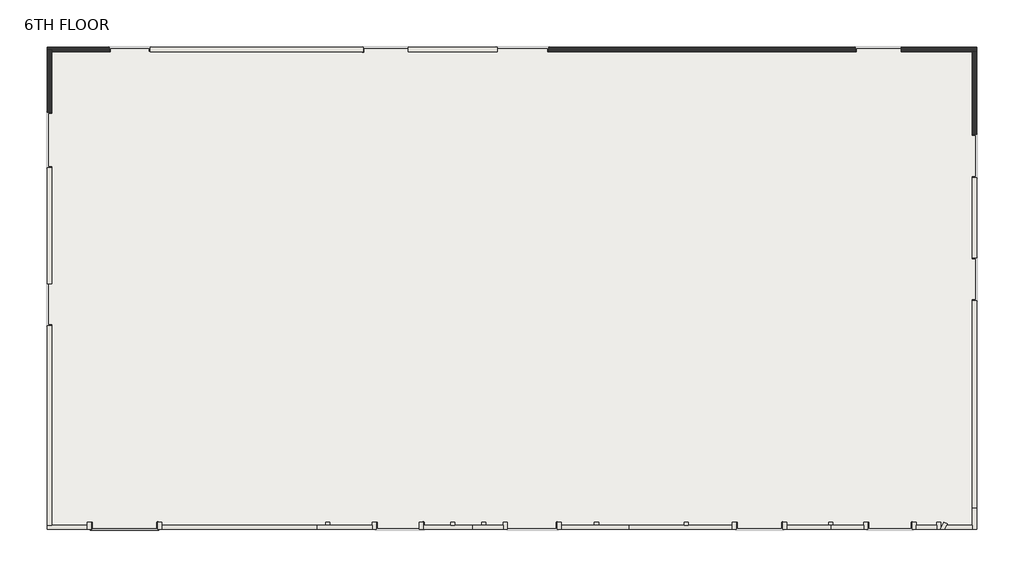
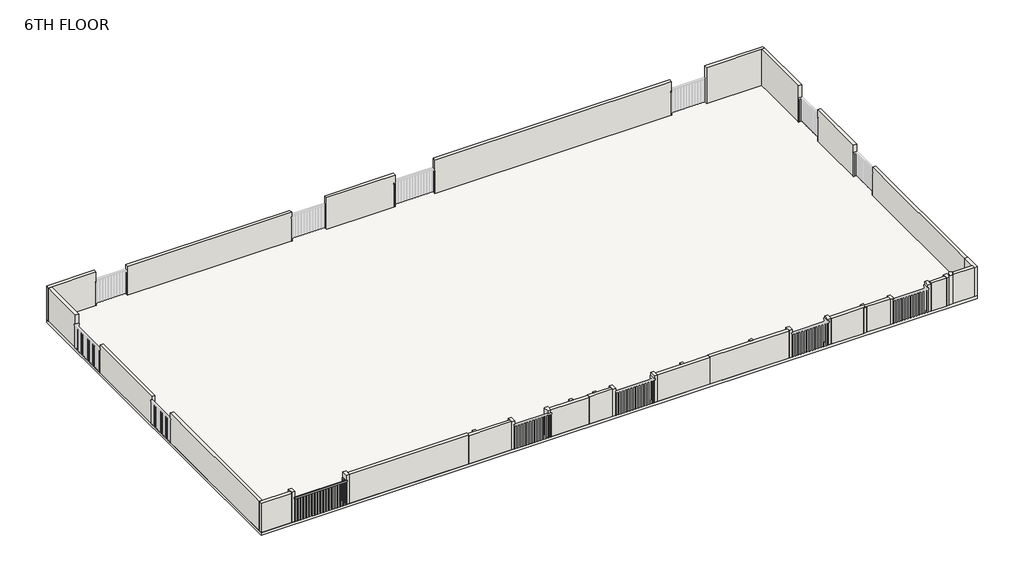
# One storey, part 1 of 3: 41 walls, 1 railing, 1 slab.
"""IFC4 building model written with IfcOpenShell, lengths in millimetres."""

from ifc_helpers import new_model, si_unit, frame, origin, place, context, project, spatial, polyline, outline, extrude, faceted_brep, element, save

model = new_model("IFC4")

# Units and contexts
model_context = context("Model", 3, world=origin())
ifc_project = project(units=[si_unit("LENGTHUNIT", "METRE", prefix="MILLI")], contexts=[model_context])

# Site, building, storey
site = spatial("IfcSite", under=ifc_project)
building = spatial("IfcBuilding", under=site)
storey = spatial("IfcBuildingStorey", under=building, Name="6TH FLOOR", Elevation=19202.4)

# Railing
placement = place(None, origin())
element("IfcRailing", 1, ObjectType="Handrail - Rectangular", at=placement, inside=storey, context=model_context, shape_type="SolidModel", body=[
    faceted_brep([(-11856.9067989, -4623.6932193, 20116.8), (-11856.9067989, -4623.6932193, 20066.0), (-11907.7067989, -4623.6932193, 20066.0), (-11907.7067989, -4623.6932193, 20116.8), (-11856.9067989, -4801.4932661, 20116.8), (-11856.9067989, -4801.4932661, 20066.0), (-11907.7067989, -4852.2932661, 20066.0), (-11907.7067989, -4852.2932661, 20116.8), (-10071.3470335, -4801.4932661, 20116.8), (-10071.3470335, -4801.4932661, 20066.0), (-10020.5470335, -4852.2932661, 20066.0), (-10020.5470335, -4852.2932661, 20116.8), (-10071.3470335, -4623.6932193, 20116.8), (-10020.5470335, -4623.6932193, 20116.8), (-10020.5470335, -4623.6932193, 20066.0), (-10071.3470335, -4623.6932193, 20066.0)], [[[0, 1, 2, 3]], [[1, 0, 4, 5]], [[2, 1, 5, 6]], [[3, 2, 6, 7]], [[0, 3, 7, 4]], [[5, 4, 8, 9]], [[6, 5, 9, 10]], [[7, 6, 10, 11]], [[4, 7, 11, 8]], [[12, 13, 14, 15]], [[9, 8, 12, 15]], [[10, 9, 15, 14]], [[11, 10, 14, 13]], [[8, 11, 13, 12]]]),
    extrude(outline(polyline([(-10036.4220335, -4633.2182661), (-10055.4720335, -4633.2182661), (-10055.4720335, -4614.1682661), (-10036.4220335, -4614.1682661), (-10036.4220335, -4633.2182661)])), frame((0.0, 0.0, 19202.4), z_axis=(0.0, 0.0, 1.0), x_axis=(1.0, 0.0, 0.0)), (0.0, 0.0, 1.0), 863.6),
    extrude(outline(polyline([(-10036.4220335, -4734.8182661), (-10055.4720335, -4734.8182661), (-10055.4720335, -4715.7682661), (-10036.4220335, -4715.7682661), (-10036.4220335, -4734.8182661)])), frame((0.0, 0.0, 19202.4), z_axis=(0.0, 0.0, 1.0), x_axis=(1.0, 0.0, 0.0)), (0.0, 0.0, 1.0), 863.6),
    extrude(outline(polyline([(-10063.0317989, -4836.4182661), (-10063.0317989, -4817.3682661), (-10043.9817989, -4817.3682661), (-10043.9817989, -4836.4182661), (-10063.0317989, -4836.4182661)])), frame((0.0, 0.0, 19202.4), z_axis=(0.0, 0.0, 1.0), x_axis=(1.0, 0.0, 0.0)), (0.0, 0.0, 1.0), 863.6),
    extrude(outline(polyline([(-10164.6317989, -4836.4182661), (-10164.6317989, -4817.3682661), (-10145.5817989, -4817.3682661), (-10145.5817989, -4836.4182661), (-10164.6317989, -4836.4182661)])), frame((0.0, 0.0, 19202.4), z_axis=(0.0, 0.0, 1.0), x_axis=(1.0, 0.0, 0.0)), (0.0, 0.0, 1.0), 863.6),
    extrude(outline(polyline([(-10266.2317989, -4836.4182661), (-10266.2317989, -4817.3682661), (-10247.1817989, -4817.3682661), (-10247.1817989, -4836.4182661), (-10266.2317989, -4836.4182661)])), frame((0.0, 0.0, 19202.4), z_axis=(0.0, 0.0, 1.0), x_axis=(1.0, 0.0, 0.0)), (0.0, 0.0, 1.0), 863.6),
    extrude(outline(polyline([(-10367.8317989, -4836.4182661), (-10367.8317989, -4817.3682661), (-10348.7817989, -4817.3682661), (-10348.7817989, -4836.4182661), (-10367.8317989, -4836.4182661)])), frame((0.0, 0.0, 19202.4), z_axis=(0.0, 0.0, 1.0), x_axis=(1.0, 0.0, 0.0)), (0.0, 0.0, 1.0), 863.6),
    extrude(outline(polyline([(-10469.4317989, -4836.4182661), (-10469.4317989, -4817.3682661), (-10450.3817989, -4817.3682661), (-10450.3817989, -4836.4182661), (-10469.4317989, -4836.4182661)])), frame((0.0, 0.0, 19202.4), z_axis=(0.0, 0.0, 1.0), x_axis=(1.0, 0.0, 0.0)), (0.0, 0.0, 1.0), 863.6),
    extrude(outline(polyline([(-10571.0317989, -4836.4182661), (-10571.0317989, -4817.3682661), (-10551.9817989, -4817.3682661), (-10551.9817989, -4836.4182661), (-10571.0317989, -4836.4182661)])), frame((0.0, 0.0, 19202.4), z_axis=(0.0, 0.0, 1.0), x_axis=(1.0, 0.0, 0.0)), (0.0, 0.0, 1.0), 863.6),
    extrude(outline(polyline([(-10672.6317989, -4836.4182661), (-10672.6317989, -4817.3682661), (-10653.5817989, -4817.3682661), (-10653.5817989, -4836.4182661), (-10672.6317989, -4836.4182661)])), frame((0.0, 0.0, 19202.4), z_axis=(0.0, 0.0, 1.0), x_axis=(1.0, 0.0, 0.0)), (0.0, 0.0, 1.0), 863.6),
    extrude(outline(polyline([(-10774.2317989, -4836.4182661), (-10774.2317989, -4817.3682661), (-10755.1817989, -4817.3682661), (-10755.1817989, -4836.4182661), (-10774.2317989, -4836.4182661)])), frame((0.0, 0.0, 19202.4), z_axis=(0.0, 0.0, 1.0), x_axis=(1.0, 0.0, 0.0)), (0.0, 0.0, 1.0), 863.6),
    extrude(outline(polyline([(-10875.8317989, -4836.4182661), (-10875.8317989, -4817.3682661), (-10856.7817989, -4817.3682661), (-10856.7817989, -4836.4182661), (-10875.8317989, -4836.4182661)])), frame((0.0, 0.0, 19202.4), z_axis=(0.0, 0.0, 1.0), x_axis=(1.0, 0.0, 0.0)), (0.0, 0.0, 1.0), 863.6),
    extrude(outline(polyline([(-10977.4317989, -4836.4182661), (-10977.4317989, -4817.3682661), (-10958.3817989, -4817.3682661), (-10958.3817989, -4836.4182661), (-10977.4317989, -4836.4182661)])), frame((0.0, 0.0, 19202.4), z_axis=(0.0, 0.0, 1.0), x_axis=(1.0, 0.0, 0.0)), (0.0, 0.0, 1.0), 863.6),
    extrude(outline(polyline([(-11079.0317989, -4836.4182661), (-11079.0317989, -4817.3682661), (-11059.9817989, -4817.3682661), (-11059.9817989, -4836.4182661), (-11079.0317989, -4836.4182661)])), frame((0.0, 0.0, 19202.4), z_axis=(0.0, 0.0, 1.0), x_axis=(1.0, 0.0, 0.0)), (0.0, 0.0, 1.0), 863.6),
    extrude(outline(polyline([(-11180.6317989, -4836.4182661), (-11180.6317989, -4817.3682661), (-11161.5817989, -4817.3682661), (-11161.5817989, -4836.4182661), (-11180.6317989, -4836.4182661)])), frame((0.0, 0.0, 19202.4), z_axis=(0.0, 0.0, 1.0), x_axis=(1.0, 0.0, 0.0)), (0.0, 0.0, 1.0), 863.6),
    extrude(outline(polyline([(-11282.2317989, -4836.4182661), (-11282.2317989, -4817.3682661), (-11263.1817989, -4817.3682661), (-11263.1817989, -4836.4182661), (-11282.2317989, -4836.4182661)])), frame((0.0, 0.0, 19202.4), z_axis=(0.0, 0.0, 1.0), x_axis=(1.0, 0.0, 0.0)), (0.0, 0.0, 1.0), 863.6),
    extrude(outline(polyline([(-11383.8317989, -4836.4182661), (-11383.8317989, -4817.3682661), (-11364.7817989, -4817.3682661), (-11364.7817989, -4836.4182661), (-11383.8317989, -4836.4182661)])), frame((0.0, 0.0, 19202.4), z_axis=(0.0, 0.0, 1.0), x_axis=(1.0, 0.0, 0.0)), (0.0, 0.0, 1.0), 863.6),
    extrude(outline(polyline([(-11485.4317989, -4836.4182661), (-11485.4317989, -4817.3682661), (-11466.3817989, -4817.3682661), (-11466.3817989, -4836.4182661), (-11485.4317989, -4836.4182661)])), frame((0.0, 0.0, 19202.4), z_axis=(0.0, 0.0, 1.0), x_axis=(1.0, 0.0, 0.0)), (0.0, 0.0, 1.0), 863.6),
    extrude(outline(polyline([(-11587.0317989, -4836.4182661), (-11587.0317989, -4817.3682661), (-11567.9817989, -4817.3682661), (-11567.9817989, -4836.4182661), (-11587.0317989, -4836.4182661)])), frame((0.0, 0.0, 19202.4), z_axis=(0.0, 0.0, 1.0), x_axis=(1.0, 0.0, 0.0)), (0.0, 0.0, 1.0), 863.6),
    extrude(outline(polyline([(-11688.6317989, -4836.4182661), (-11688.6317989, -4817.3682661), (-11669.5817989, -4817.3682661), (-11669.5817989, -4836.4182661), (-11688.6317989, -4836.4182661)])), frame((0.0, 0.0, 19202.4), z_axis=(0.0, 0.0, 1.0), x_axis=(1.0, 0.0, 0.0)), (0.0, 0.0, 1.0), 863.6),
    extrude(outline(polyline([(-11790.2317989, -4836.4182661), (-11790.2317989, -4817.3682661), (-11771.1817989, -4817.3682661), (-11771.1817989, -4836.4182661), (-11790.2317989, -4836.4182661)])), frame((0.0, 0.0, 19202.4), z_axis=(0.0, 0.0, 1.0), x_axis=(1.0, 0.0, 0.0)), (0.0, 0.0, 1.0), 863.6),
    extrude(outline(polyline([(-11891.8317989, -4817.3682193), (-11872.7817989, -4817.3682193), (-11872.7817989, -4836.4182193), (-11891.8317989, -4836.4182193), (-11891.8317989, -4817.3682193)])), frame((0.0, 0.0, 19202.4), z_axis=(0.0, 0.0, 1.0), x_axis=(1.0, 0.0, 0.0)), (0.0, 0.0, 1.0), 863.6),
    extrude(outline(polyline([(-11891.8317989, -4715.7682193), (-11872.7817989, -4715.7682193), (-11872.7817989, -4734.8182193), (-11891.8317989, -4734.8182193), (-11891.8317989, -4715.7682193)])), frame((0.0, 0.0, 19202.4), z_axis=(0.0, 0.0, 1.0), x_axis=(1.0, 0.0, 0.0)), (0.0, 0.0, 1.0), 863.6),
    extrude(outline(polyline([(-10055.4720335, -4836.4182661), (-10055.4720335, -4817.3682661), (-10036.4220335, -4817.3682661), (-10036.4220335, -4836.4182661), (-10055.4720335, -4836.4182661)])), frame((0.0, 0.0, 19202.4), z_axis=(0.0, 0.0, 1.0), x_axis=(1.0, 0.0, 0.0)), (0.0, 0.0, 1.0), 863.6),
    extrude(outline(polyline([(-11891.8317989, -4817.3682661), (-11872.7817989, -4817.3682661), (-11872.7817989, -4836.4182661), (-11891.8317989, -4836.4182661), (-11891.8317989, -4817.3682661)])), frame((0.0, 0.0, 19202.4), z_axis=(0.0, 0.0, 1.0), x_axis=(1.0, 0.0, 0.0)), (0.0, 0.0, 1.0), 863.6),
    extrude(outline(polyline([(-10036.4220335, -4642.7432193), (-10055.4720335, -4642.7432193), (-10055.4720335, -4623.6932193), (-10036.4220335, -4623.6932193), (-10036.4220335, -4642.7432193)])), frame((0.0, 0.0, 19202.4), z_axis=(0.0, 0.0, 1.0), x_axis=(1.0, 0.0, 0.0)), (0.0, 0.0, 1.0), 863.6),
    extrude(outline(polyline([(-11891.8317989, -4623.6932193), (-11872.7817989, -4623.6932193), (-11872.7817989, -4642.7432193), (-11891.8317989, -4642.7432193), (-11891.8317989, -4623.6932193)])), frame((0.0, 0.0, 19202.4), z_axis=(0.0, 0.0, 1.0), x_axis=(1.0, 0.0, 0.0)), (0.0, 0.0, 1.0), 863.6),
])

# Slab
element("IfcSlab", 2, ObjectType="LW Concrete on Metal Deck", at=placement, inside=storey, context=model_context, shape_type="SweptSolid", body=[
    extrude(outline(polyline([(12540.3012043, 8470.0067329), (12540.3012043, -4826.8932661), (-13088.8067989, -4826.8932661), (-13088.8067989, 8470.0067329), (12540.3012043, 8470.0067329)])), frame((0.0, 0.0, 19097.625), z_axis=(0.0, 0.0, 1.0), x_axis=(1.0, 0.0, 0.0)), (0.0, 0.0, 1.0), 104.775),
])

# Walls
element("IfcWall", 3, ObjectType="Generic - 4.5\"", at=placement, inside=storey, context=model_context, shape_type="Brep", body=[
    faceted_brep([(-13088.8067989, -4826.8932661, 19202.4), (-11996.6067989, -4826.8932661, 19202.4), (-11996.6067989, -4826.8932661, 20315.3417562), (-13088.8067989, -4826.8932661, 20315.3417562), (-13088.8067989, -4712.5932661, 19202.4), (-13088.8067989, -4712.5932661, 20315.3417562), (-11996.6067989, -4712.5932661, 20315.3417562), (-11996.6067989, -4712.5932661, 19202.4), (-12974.5067989, -4712.5932661, 19202.4)], [[[0, 1, 2, 3]], [[4, 5, 6, 7, 8]], [[1, 0, 4, 8, 7]], [[3, 2, 6, 5]], [[2, 1, 7, 6]], [[0, 3, 5, 4]]]),
])
element("IfcWall", 4, ObjectType="Generic - 4.5\"", at=placement, inside=storey, context=model_context, shape_type="Brep", body=[
    faceted_brep([(-11996.6067989, -4623.6932193, 19202.4), (-11996.6067989, -4712.5932661, 19202.4), (-11996.6067989, -4826.8932661, 19202.4), (-11996.6067989, -4826.8932661, 20315.3417562), (-11996.6067989, -4826.8932661, 20336.3303619), (-11996.6067989, -4623.6932193, 20336.3303619), (-11882.3067989, -4623.6932193, 19202.4), (-11882.3067989, -4623.6932193, 20336.3303619), (-11882.3067989, -4826.8932661, 20336.3303619), (-11882.3067989, -4826.8932661, 19202.4)], [[[0, 1, 2, 3, 4, 5]], [[6, 7, 8, 9]], [[2, 1, 0, 6, 9]], [[5, 4, 8, 7]], [[0, 5, 7, 6]], [[4, 3, 2, 9, 8]]]),
])
element("IfcWall", 5, ObjectType="Generic - 4.5\"", at=placement, inside=storey, context=model_context, shape_type="Brep", body=[
    faceted_brep([(11660.3143245, -4826.8932661, 19202.4), (12426.0012043, -4826.8932661, 19202.4), (12426.0012043, -4826.8932661, 20294.2617784), (12426.0012043, -4826.8932661, 20305.5196614), (11660.3143245, -4826.8932661, 20305.5196614), (11660.3143245, -4826.8932661, 20291.9342527), (11716.0621594, -4712.5932661, 19202.4), (11716.0621594, -4712.5932661, 20305.5196614), (12426.0012043, -4712.5932661, 20305.5196614), (12426.0012043, -4712.5932661, 19202.4)], [[[0, 1, 2, 3, 4, 5]], [[6, 7, 8, 9]], [[1, 0, 6, 9]], [[4, 3, 8, 7]], [[3, 2, 1, 9, 8]], [[0, 5, 4, 7, 6]]]),
])
element("IfcWall", 6, ObjectType="Generic - 4.5\"", at=placement, inside=storey, context=model_context, shape_type="Brep", body=[
    faceted_brep([(11632.2512075, -4623.6932193, 19202.4), (11533.1439227, -4826.8932661, 19202.4), (11533.1439227, -4826.8932661, 20291.9342527), (11632.2512075, -4623.6932193, 20291.9342527), (11734.983367, -4673.7990414, 19202.4), (11734.983367, -4673.7990414, 20291.9342527), (11660.3143245, -4826.8932661, 20291.9342527), (11660.3143245, -4826.8932661, 19202.4), (11716.0621594, -4712.5932661, 19202.4)], [[[0, 1, 2, 3]], [[4, 5, 6, 7, 8]], [[1, 0, 4, 8, 7]], [[3, 2, 6, 5]], [[0, 3, 5, 4]], [[2, 1, 7, 6]]]),
])
element("IfcWall", 7, ObjectType="Generic - 4.5\"", at=placement, inside=storey, context=model_context, shape_type="Brep", body=[
    faceted_brep([(12426.0012043, -4236.3432661, 19202.4), (12426.0012043, -4712.5932661, 19202.4), (12426.0012043, -4826.8932661, 19202.4), (12426.0012043, -4826.8932661, 20294.2617784), (12426.0012043, -4236.3432661, 20294.2617784), (12426.0012043, -4236.3432661, 20289.0712164), (12540.3012043, -4236.3432661, 19202.4), (12540.3012043, -4236.3432661, 20289.0712164), (12540.3012043, -4236.3432661, 20294.2617784), (12540.3012043, -4826.8932661, 20294.2617784), (12540.3012043, -4826.8932661, 19202.4)], [[[0, 1, 2, 3, 4, 5]], [[6, 7, 8, 9, 10]], [[2, 1, 0, 6, 10]], [[4, 3, 9, 8]], [[0, 5, 4, 8, 7, 6]], [[3, 2, 10, 9]]]),
])
element("IfcWall", 8, ObjectType="Generic - 4.5\"", at=placement, inside=storey, context=model_context, shape_type="SweptSolid", body=[
    extrude(outline(polyline([(-5417.4987995, -4712.5932661), (-5417.4987995, -4623.6932193), (-5303.1987995, -4623.6932193), (-5303.1987995, -4712.5932661), (-5417.4987995, -4712.5932661)])), frame((0.0, 0.0, 19202.4), z_axis=(0.0, 0.0, 1.0), x_axis=(1.0, 0.0, 0.0)), (0.0, 0.0, 1.0), 1063.0786215),
])
element("IfcWall", 9, ObjectType="Generic - 4.5\"", at=placement, inside=storey, context=model_context, shape_type="Brep", body=[
    faceted_brep([(-5663.8033402, -4826.8932661, 19202.4), (-4134.7987995, -4826.8932661, 19202.4), (-4134.7987995, -4826.8932661, 20261.5218247), (-4134.7987995, -4826.8932661, 20269.6575049), (-5663.8033402, -4826.8932661, 20269.6575049), (-5663.8033402, -4712.5932661, 19202.4), (-5663.8033402, -4712.5932661, 20269.6575049), (-4134.7987995, -4712.5932661, 20269.6575049), (-4134.7987995, -4712.5932661, 19202.4), (-5303.1987995, -4712.5932661, 19202.4), (-5417.4987995, -4712.5932661, 19202.4)], [[[0, 1, 2, 3, 4]], [[5, 6, 7, 8, 9, 10]], [[1, 0, 5, 10, 9, 8]], [[4, 3, 7, 6]], [[0, 4, 6, 5]], [[3, 2, 1, 8, 7]]]),
])
element("IfcWall", 10, ObjectType="Generic - 4.5\"", at=placement, inside=storey, context=model_context, shape_type="Brep", body=[
    faceted_brep([(-2725.0987995, -4826.8932661, 19202.4), (-1354.4417672, -4826.8932661, 19202.4), (-1354.4417672, -4826.8932661, 20218.4), (-2725.0987995, -4826.8932661, 20218.4), (-2725.0987995, -4712.5932661, 19202.4), (-2725.0987995, -4712.5932661, 20218.4), (-1354.4417672, -4712.5932661, 20218.4), (-1354.4417672, -4712.5932661, 19202.4), (-1848.7987998, -4712.5932661, 19202.4), (-1963.0987998, -4712.5932661, 19202.4)], [[[0, 1, 2, 3]], [[4, 5, 6, 7, 8, 9]], [[1, 0, 4, 9, 8, 7]], [[2, 1, 7, 6]], [[3, 2, 6, 5]], [[0, 3, 5, 4]]]),
])
element("IfcWall", 11, ObjectType="Generic - 4.5\"", at=placement, inside=storey, context=model_context, shape_type="SweptSolid", body=[
    extrude(outline(polyline([(-1963.0987998, -4712.5932661), (-1963.0987998, -4623.6932193), (-1848.7987998, -4623.6932193), (-1848.7987998, -4712.5932661), (-1963.0987998, -4712.5932661)])), frame((0.0, 0.0, 19202.4), z_axis=(0.0, 0.0, 1.0), x_axis=(1.0, 0.0, 0.0)), (0.0, 0.0, 1.0), 1029.3234006),
])
element("IfcWall", 12, ObjectType="Generic - 4.5\"", at=placement, inside=storey, context=model_context, shape_type="SweptSolid", body=[
    extrude(outline(polyline([(-1112.1987998, -4712.5932661), (-1112.1987998, -4623.6932193), (-997.8987998, -4623.6932193), (-997.8987998, -4712.5932661), (-1112.1987998, -4712.5932661)])), frame((0.0, 0.0, 19202.4), z_axis=(0.0, 0.0, 1.0), x_axis=(1.0, 0.0, 0.0)), (0.0, 0.0, 1.0), 1016.0),
])
element("IfcWall", 13, ObjectType="Generic - 4.5\"", at=placement, inside=storey, context=model_context, shape_type="SweptSolid", body=[
    extrude(outline(polyline([(1999.3012002, -4712.5932661), (1999.3012002, -4623.6932193), (2113.6012002, -4623.6932193), (2113.6012002, -4712.5932661), (1999.3012002, -4712.5932661)])), frame((0.0, 0.0, 19202.4), z_axis=(0.0, 0.0, 1.0), x_axis=(1.0, 0.0, 0.0)), (0.0, 0.0, 1.0), 1013.2250283),
])
element("IfcWall", 14, ObjectType="Generic - 4.5\"", at=placement, inside=storey, context=model_context, shape_type="SweptSolid", body=[
    extrude(outline(polyline([(4475.8012082, -4712.5932661), (4475.8012082, -4623.6932193), (4590.1012082, -4623.6932193), (4590.1012082, -4712.5932661), (4475.8012082, -4712.5932661)])), frame((0.0, 0.0, 19202.4), z_axis=(0.0, 0.0, 1.0), x_axis=(1.0, 0.0, 0.0)), (0.0, 0.0, 1.0), 1027.4591445),
])
element("IfcWall", 15, ObjectType="Generic - 4.5\"", at=placement, inside=storey, context=model_context, shape_type="Brep", body=[
    faceted_brep([(2962.6087812, -4826.8932661, 19202.4), (5802.9512082, -4826.8932661, 19202.4), (5802.9512082, -4826.8932661, 20229.8591445), (2962.6087812, -4826.8932661, 20229.8591445), (2962.6087812, -4826.8932661, 20215.6250283), (2962.6087812, -4712.5932661, 19202.4), (2962.6087812, -4712.5932661, 20215.6250283), (2962.6087812, -4712.5932661, 20229.8591445), (4475.8012082, -4712.5932661, 20229.8591445), (4590.1012082, -4712.5932661, 20229.8591445), (5802.9512082, -4712.5932661, 20229.8591445), (5802.9512082, -4712.5932661, 19202.4), (4590.1012082, -4712.5932661, 19202.4), (4475.8012082, -4712.5932661, 19202.4)], [[[0, 1, 2, 3, 4]], [[5, 6, 7, 8, 9, 10, 11, 12, 13]], [[1, 0, 5, 13, 12, 11]], [[3, 2, 10, 9, 8, 7]], [[0, 4, 3, 7, 6, 5]], [[2, 1, 11, 10]]]),
])
element("IfcWall", 16, ObjectType="Generic - 4.5\"", at=placement, inside=storey, context=model_context, shape_type="Brep", body=[
    faceted_brep([(5802.9512082, -4623.6932193, 19202.4), (5802.9512082, -4712.5932661, 19202.4), (5802.9512082, -4826.8932661, 19202.4), (5802.9512082, -4826.8932661, 20229.8591445), (5802.9512082, -4826.8932661, 20234.7822201), (5802.9512082, -4623.6932193, 20234.7822201), (5917.2512082, -4623.6932193, 19202.4), (5917.2512082, -4623.6932193, 20234.7822201), (5917.2512082, -4826.8932661, 20234.7822201), (5917.2512082, -4826.8932661, 19202.4)], [[[0, 1, 2, 3, 4, 5]], [[6, 7, 8, 9]], [[2, 1, 0, 6, 9]], [[5, 4, 8, 7]], [[0, 5, 7, 6]], [[4, 3, 2, 9, 8]]]),
])
element("IfcWall", 17, ObjectType="Generic - 4.5\"", at=placement, inside=storey, context=model_context, shape_type="Brep", body=[
    faceted_brep([(7190.3011643, -4623.6932193, 19202.4), (7190.3011643, -4826.8932661, 19202.4), (7190.3011643, -4826.8932661, 20175.2158009), (7190.3011643, -4623.6932193, 20175.2158009), (7304.6011643, -4623.6932193, 19202.4), (7304.6011643, -4623.6932193, 20175.2158009), (7304.6011643, -4712.5932661, 20175.2158009), (7304.6011643, -4826.8932661, 20175.2158009), (7304.6011643, -4826.8932661, 19202.4), (7304.6011643, -4712.5932661, 19202.4)], [[[0, 1, 2, 3]], [[4, 5, 6, 7, 8, 9]], [[1, 0, 4, 9, 8]], [[3, 2, 7, 6, 5]], [[0, 3, 5, 4]], [[2, 1, 8, 7]]]),
])
element("IfcWall", 18, ObjectType="Generic - 4.5\"", at=placement, inside=storey, context=model_context, shape_type="Brep", body=[
    faceted_brep([(7304.6011643, -4826.8932661, 19202.4), (8463.6012082, -4826.8932661, 19202.4), (8463.6012082, -4826.8932661, 20158.8159658), (8520.7512082, -4826.8932661, 20158.8159658), (8520.7512082, -4826.8932661, 20172.080309), (8520.7512082, -4826.8932661, 20175.3581334), (7304.6011643, -4826.8932661, 20175.3581334), (7304.6011643, -4712.5932661, 19202.4), (7304.6011643, -4712.5932661, 20175.3581334), (8520.7512082, -4712.5932661, 20175.3581334), (8520.7512082, -4712.5932661, 20172.080309), (8520.7512082, -4712.5932661, 20158.8159658), (8463.6012082, -4712.5932661, 20158.8159658), (8463.6012082, -4712.5932661, 19202.4)], [[[0, 1, 2, 3, 4, 5, 6]], [[7, 8, 9, 10, 11, 12, 13]], [[1, 0, 7, 13]], [[6, 5, 9, 8]], [[0, 6, 8, 7]], [[5, 4, 3, 11, 10, 9]], [[11, 3, 2, 12]], [[2, 1, 13, 12]]]),
])
element("IfcWall", 19, ObjectType="Generic - 4.5\"", at=placement, inside=storey, context=model_context, shape_type="Brep", body=[
    faceted_brep([(8463.6012082, -4623.6932193, 19202.4), (8463.6012082, -4712.5932661, 19202.4), (8463.6012082, -4826.8932661, 19202.4), (8463.6012082, -4826.8932661, 20158.8159658), (8463.6012082, -4712.5932661, 20158.8159658), (8463.6012082, -4623.6932193, 20158.8159658), (8577.9012082, -4623.6932193, 19202.4), (8577.9012082, -4623.6932193, 20158.8159658), (8577.9012082, -4712.5932661, 20158.8159658), (8577.9012082, -4826.8932661, 20158.8159658), (8577.9012082, -4826.8932661, 19202.4), (8577.9012082, -4712.5932661, 19202.4), (8520.7512082, -4826.8932661, 20158.8159658)], [[[0, 1, 2, 3, 4, 5]], [[6, 7, 8, 9, 10, 11]], [[2, 1, 0, 6, 11, 10]], [[5, 4, 3, 12, 9, 8, 7]], [[0, 5, 7, 6]], [[3, 2, 10, 9, 12]]]),
])
element("IfcWall", 20, ObjectType="Generic - 4.5\"", at=placement, inside=storey, context=model_context, shape_type="Brep", body=[
    faceted_brep([(8577.9012082, -4826.8932661, 19202.4), (9422.4512082, -4826.8932661, 19202.4), (9422.4512082, -4826.8932661, 20154.6060641), (9422.4512082, -4826.8932661, 20172.080309), (8520.7512082, -4826.8932661, 20172.080309), (8520.7512082, -4826.8932661, 20158.8159658), (8577.9012082, -4826.8932661, 20158.8159658), (8577.9012082, -4712.5932661, 19202.4), (8577.9012082, -4712.5932661, 20158.8159658), (8520.7512082, -4712.5932661, 20158.8159658), (8520.7512082, -4712.5932661, 20172.080309), (9422.4512082, -4712.5932661, 20172.080309), (9422.4512082, -4712.5932661, 19202.4)], [[[0, 1, 2, 3, 4, 5, 6]], [[7, 8, 9, 10, 11, 12]], [[1, 0, 7, 12]], [[4, 3, 11, 10]], [[3, 2, 1, 12, 11]], [[5, 4, 10, 9]], [[5, 9, 8, 6]], [[0, 6, 8, 7]]]),
])
element("IfcWall", 21, ObjectType="Generic - 4.5\"", at=placement, inside=storey, context=model_context, shape_type="Brep", body=[
    faceted_brep([(9422.4512082, -4623.6932193, 19202.4), (9422.4512082, -4712.5932661, 19202.4), (9422.4512082, -4826.8932661, 19202.4), (9422.4512082, -4826.8932661, 20154.6060641), (9422.4512082, -4623.6932193, 20154.6060641), (9536.7512082, -4623.6932193, 19202.4), (9536.7512082, -4623.6932193, 20154.6060641), (9536.7512082, -4826.8932661, 20154.6060641), (9536.7512082, -4826.8932661, 19202.4)], [[[0, 1, 2, 3, 4]], [[5, 6, 7, 8]], [[2, 1, 0, 5, 8]], [[4, 3, 7, 6]], [[0, 4, 6, 5]], [[3, 2, 8, 7]]]),
])
element("IfcWall", 22, ObjectType="Generic - 4.5\"", at=placement, inside=storey, context=model_context, shape_type="Brep", body=[
    faceted_brep([(10764.1617205, -4623.6932193, 19202.4), (10764.1617205, -4826.8932661, 19202.4), (10764.1617205, -4826.8932661, 20228.7072304), (10764.1617205, -4623.6932193, 20228.7072304), (10878.4617205, -4623.6932193, 19202.4), (10878.4617205, -4623.6932193, 20228.7072304), (10878.4617205, -4826.8932661, 20228.7072304), (10878.4617205, -4826.8932661, 19202.4), (10878.4617205, -4712.5932661, 19202.4)], [[[0, 1, 2, 3]], [[4, 5, 6, 7, 8]], [[1, 0, 4, 8, 7]], [[3, 2, 6, 5]], [[0, 3, 5, 4]], [[2, 1, 7, 6]]]),
])
element("IfcWall", 23, ObjectType="Generic - 4.5\"", at=placement, inside=storey, context=model_context, shape_type="Brep", body=[
    faceted_brep([(10878.4617205, -4826.8932661, 19202.4), (11437.2617205, -4826.8932661, 19202.4), (11437.2617205, -4826.8932661, 20251.0912221), (10878.4617205, -4826.8932661, 20251.0912221), (10878.4617205, -4826.8932661, 20228.7072304), (10878.4617205, -4712.5932661, 19202.4), (10878.4617205, -4712.5932661, 20251.0912221), (11437.2617205, -4712.5932661, 20251.0912221), (11437.2617205, -4712.5932661, 19202.4)], [[[0, 1, 2, 3, 4]], [[5, 6, 7, 8]], [[1, 0, 5, 8]], [[3, 2, 7, 6]], [[0, 4, 3, 6, 5]], [[2, 1, 8, 7]]]),
])
element("IfcWall", 24, ObjectType="Generic - 4.5\"", at=placement, inside=storey, context=model_context, shape_type="Brep", body=[
    faceted_brep([(11437.2617205, -4623.6932193, 19202.4), (11437.2617205, -4712.5932661, 19202.4), (11437.2617205, -4826.8932661, 19202.4), (11437.2617205, -4826.8932661, 20251.0912221), (11437.2617205, -4712.5932661, 20251.0912221), (11437.2617205, -4623.6932193, 20251.0912221), (11551.5617205, -4623.6932193, 19202.4), (11551.5617205, -4623.6932193, 20251.0912221), (11551.5617205, -4826.8932661, 20251.0912221), (11551.5617205, -4826.8932661, 19202.4)], [[[0, 1, 2, 3, 4, 5]], [[6, 7, 8, 9]], [[2, 1, 0, 6, 9]], [[5, 4, 3, 8, 7]], [[0, 5, 7, 6]], [[3, 2, 9, 8]]]),
])
element("IfcWall", 25, ObjectType="Generic - 4.5\"", at=placement, inside=storey, context=model_context, shape_type="Brep", body=[
    faceted_brep([(-4134.7987995, -4623.6932193, 19202.4), (-4134.7987995, -4712.5932661, 19202.4), (-4134.7987995, -4826.8932661, 19202.4), (-4134.7987995, -4826.8932661, 20261.5218247), (-4134.7987995, -4623.6932193, 20261.5218247), (-4020.4987995, -4623.6932193, 19202.4), (-4020.4987995, -4623.6932193, 20261.5218247), (-4020.4987995, -4826.8932661, 20261.5218247), (-4020.4987995, -4826.8932661, 19202.4)], [[[0, 1, 2, 3, 4]], [[5, 6, 7, 8]], [[2, 1, 0, 5, 8]], [[4, 3, 7, 6]], [[0, 4, 6, 5]], [[3, 2, 8, 7]]]),
])
element("IfcWall", 26, ObjectType="Generic - 4.5\"", at=placement, inside=storey, context=model_context, shape_type="Brep", body=[
    faceted_brep([(-2839.3987995, -4623.6932193, 19202.4), (-2839.3987995, -4826.8932661, 19202.4), (-2839.3987995, -4826.8932661, 20219.1549618), (-2839.3987995, -4623.6932193, 20219.1549618), (-2725.0987995, -4623.6932193, 19202.4), (-2725.0987995, -4623.6932193, 20219.1549618), (-2725.0987995, -4826.8932661, 20219.1549618), (-2725.0987995, -4826.8932661, 20218.4), (-2725.0987995, -4826.8932661, 19202.4), (-2725.0987995, -4712.5932661, 19202.4)], [[[0, 1, 2, 3]], [[4, 5, 6, 7, 8, 9]], [[1, 0, 4, 9, 8]], [[3, 2, 6, 5]], [[0, 3, 5, 4]], [[2, 1, 8, 7, 6]]]),
])
element("IfcWall", 27, ObjectType="Generic - 4.5\"", at=placement, inside=storey, context=model_context, shape_type="Brep", body=[
    faceted_brep([(-1354.4417672, -4826.8932661, 19202.4), (-520.5065315, -4826.8932661, 19202.4), (-520.5065315, -4826.8932661, 20226.2796817), (-520.5065315, -4826.8932661, 20233.540074), (-1354.4417672, -4826.8932661, 20233.540074), (-1354.4417672, -4826.8932661, 20218.4), (-1354.4417672, -4712.5932661, 19202.4), (-1354.4417672, -4712.5932661, 20218.4), (-1354.4417672, -4712.5932661, 20233.540074), (-520.5065315, -4712.5932661, 20233.540074), (-520.5065315, -4712.5932661, 19202.4), (-997.8987998, -4712.5932661, 19202.4), (-1112.1987998, -4712.5932661, 19202.4)], [[[0, 1, 2, 3, 4, 5]], [[6, 7, 8, 9, 10, 11, 12]], [[1, 0, 6, 12, 11, 10]], [[4, 3, 9, 8]], [[0, 5, 4, 8, 7, 6]], [[3, 2, 1, 10, 9]]]),
])
element("IfcWall", 28, ObjectType="Generic - 4.5\"", at=placement, inside=storey, context=model_context, shape_type="Brep", body=[
    faceted_brep([(-520.5065315, -4623.6932193, 19202.4), (-520.5065315, -4712.5932661, 19202.4), (-520.5065315, -4826.8932661, 19202.4), (-520.5065315, -4826.8932661, 20226.2796817), (-520.5065315, -4623.6932193, 20226.2796817), (-406.2065315, -4623.6932193, 19202.4), (-406.2065315, -4623.6932193, 20226.2796817), (-406.2065315, -4826.8932661, 20226.2796817), (-406.2065315, -4826.8932661, 19202.4)], [[[0, 1, 2, 3, 4]], [[5, 6, 7, 8]], [[2, 1, 0, 5, 8]], [[4, 3, 7, 6]], [[0, 4, 6, 5]], [[3, 2, 8, 7]]]),
])
element("IfcWall", 29, ObjectType="Generic - 4.5\"", at=placement, inside=storey, context=model_context, shape_type="Brep", body=[
    faceted_brep([(970.0932011, -4623.6932193, 19202.4), (970.0932011, -4826.8932661, 19202.4), (970.0932011, -4826.8932661, 20215.6250283), (970.0932011, -4623.6932193, 20215.6250283), (1084.3932011, -4623.6932193, 19202.4), (1084.3932011, -4623.6932193, 20215.6250283), (1084.3932011, -4712.5932661, 20215.6250283), (1084.3932011, -4826.8932661, 20215.6250283), (1084.3932011, -4826.8932661, 19202.4), (1084.3932011, -4712.5932661, 19202.4)], [[[0, 1, 2, 3]], [[4, 5, 6, 7, 8, 9]], [[1, 0, 4, 9, 8]], [[3, 2, 7, 6, 5]], [[0, 3, 5, 4]], [[2, 1, 8, 7]]]),
])
element("IfcWall", 30, ObjectType="Generic - 4.5\"", at=placement, inside=storey, context=model_context, shape_type="Brep", body=[
    faceted_brep([(1084.3932011, -4826.8932661, 19202.4), (2962.6087812, -4826.8932661, 19202.4), (2962.6087812, -4826.8932661, 20215.6250283), (1084.3932011, -4826.8932661, 20215.6250283), (1084.3932011, -4712.5932661, 19202.4), (1084.3932011, -4712.5932661, 20215.6250283), (1999.3012002, -4712.5932661, 20215.6250283), (2113.6012002, -4712.5932661, 20215.6250283), (2962.6087812, -4712.5932661, 20215.6250283), (2962.6087812, -4712.5932661, 19202.4), (2113.6012002, -4712.5932661, 19202.4), (1999.3012002, -4712.5932661, 19202.4)], [[[0, 1, 2, 3]], [[4, 5, 6, 7, 8, 9, 10, 11]], [[1, 0, 4, 11, 10, 9]], [[2, 1, 9, 8]], [[3, 2, 8, 7, 6, 5]], [[0, 3, 5, 4]]]),
])
element("IfcWall", 31, ObjectType="Generic - 4.5\"", at=placement, inside=storey, context=model_context, shape_type="Brep", body=[
    faceted_brep([(-10045.9470335, -4623.6932193, 19202.4), (-10045.9470335, -4826.8932661, 19202.4), (-10045.9470335, -4826.8932661, 20310.104535), (-10045.9470335, -4623.6932193, 20310.104535), (-9931.6470335, -4623.6932193, 19202.4), (-9931.6470335, -4623.6932193, 20310.104535), (-9931.6470335, -4712.5932661, 20310.104535), (-9931.6470335, -4826.8932661, 20310.104535), (-9931.6470335, -4826.8932661, 19202.4), (-9931.6470335, -4712.5932661, 19202.4)], [[[0, 1, 2, 3]], [[4, 5, 6, 7, 8, 9]], [[1, 0, 4, 9, 8]], [[3, 2, 7, 6, 5]], [[0, 3, 5, 4]], [[2, 1, 8, 7]]]),
])
element("IfcWall", 32, ObjectType="Generic - 4.5\"", at=placement, inside=storey, context=model_context, shape_type="Brep", body=[
    faceted_brep([(-9931.6470335, -4826.8932661, 19202.4), (-5663.8033402, -4826.8932661, 19202.4), (-5663.8033402, -4826.8932661, 20269.6575049), (-5663.8033402, -4826.8932661, 20310.104535), (-9931.6470335, -4826.8932661, 20310.104535), (-9931.6470335, -4712.5932661, 19202.4), (-9931.6470335, -4712.5932661, 20310.104535), (-5663.8033402, -4712.5932661, 20310.104535), (-5663.8033402, -4712.5932661, 20269.6575049), (-5663.8033402, -4712.5932661, 19202.4)], [[[0, 1, 2, 3, 4]], [[5, 6, 7, 8, 9]], [[1, 0, 5, 9]], [[3, 2, 1, 9, 8, 7]], [[4, 3, 7, 6]], [[0, 4, 6, 5]]]),
])
element("IfcWall", 33, ObjectType="Generic - 4.5\"", at=placement, inside=storey, context=model_context, shape_type="Brep", body=[
    faceted_brep([(-13088.8067989, 792.8567339, 19202.4), (-13088.8067989, -4712.5932661, 19202.4), (-13088.8067989, -4712.5932661, 20315.3417562), (-13088.8067989, -4712.5932661, 20316.567936), (-13088.8067989, 792.8567339, 20316.567936), (-12974.5067989, 792.8567339, 19202.4), (-12974.5067989, 792.8567339, 20316.567936), (-12974.5067989, -4712.5932661, 20316.567936), (-12974.5067989, -4712.5932661, 19202.4)], [[[0, 1, 2, 3, 4]], [[5, 6, 7, 8]], [[1, 0, 5, 8]], [[4, 3, 7, 6]], [[0, 4, 6, 5]], [[3, 2, 1, 8, 7]]]),
])
element("IfcWall", 34, ObjectType="Generic - 4.5\"", at=placement, inside=storey, context=model_context, shape_type="SweptSolid", body=[
    extrude(outline(polyline([(-12976.0338648, 5154.3604213), (-12976.0338648, 1953.9604213), (-13090.3338648, 1953.9604213), (-13090.3338648, 5154.3604213), (-12976.0338648, 5154.3604213)])), frame((0.0, 0.0, 19202.4), z_axis=(0.0, 0.0, 1.0), x_axis=(1.0, 0.0, 0.0)), (0.0, 0.0, 1.0), 1047.4413329),
])
element("IfcWall", 35, ObjectType="Generic - 4.5\"", at=placement, inside=storey, context=model_context, shape_type="SweptSolid", body=[
    extrude(outline(polyline([(-12973.9987925, 8412.8567329), (-12973.9987925, 6682.2711337), (-13088.2987925, 6682.2711337), (-13088.2987925, 8412.8567329), (-12973.9987925, 8412.8567329)])), frame((0.0, 0.0, 19202.4), z_axis=(0.0, 0.0, 1.0), x_axis=(1.0, 0.0, 0.0)), (0.0, 0.0, 1.0), 1259.0059812),
])
element("IfcWall", 36, ObjectType="Generic - 4.5\"", at=placement, inside=storey, context=model_context, shape_type="SweptSolid", body=[
    extrude(outline(polyline([(-11387.0067989, 8355.7067329), (-13088.8067989, 8355.7067329), (-13088.8067989, 8470.0067329), (-11387.0067989, 8470.0067329), (-11387.0067989, 8355.7067329)])), frame((0.0, 0.0, 19202.4), z_axis=(0.0, 0.0, 1.0), x_axis=(1.0, 0.0, 0.0)), (0.0, 0.0, 1.0), 1273.4134002),
])
element("IfcWall", 37, ObjectType="Generic - 4.5\"", at=placement, inside=storey, context=model_context, shape_type="SweptSolid", body=[
    extrude(outline(polyline([(-4382.4487992, 8355.7067329), (-10247.1817989, 8355.7067329), (-10247.1817989, 8470.0067329), (-4382.4487992, 8470.0067329), (-4382.4487992, 8355.7067329)])), frame((0.0, 0.0, 19202.4), z_axis=(0.0, 0.0, 1.0), x_axis=(1.0, 0.0, 0.0)), (0.0, 0.0, 1.0), 1083.89837),
])
element("IfcWall", 38, ObjectType="Generic - 4.5\"", at=placement, inside=storey, context=model_context, shape_type="SweptSolid", body=[
    extrude(outline(polyline([(-682.0490672, 8355.7067329), (-3139.4990672, 8355.7067329), (-3139.4990672, 8470.0067329), (-682.0490672, 8470.0067329), (-682.0490672, 8355.7067329)])), frame((0.0, 0.0, 19202.4), z_axis=(0.0, 0.0, 1.0), x_axis=(1.0, 0.0, 0.0)), (0.0, 0.0, 1.0), 1195.9732529),
])
element("IfcWall", 39, ObjectType="Generic - 4.5\"", at=placement, inside=storey, context=model_context, shape_type="SweptSolid", body=[
    extrude(outline(polyline([(9199.6932011, 8355.7067329), (741.4932011, 8355.7067329), (741.4932011, 8470.0067329), (9199.6932011, 8470.0067329), (9199.6932011, 8355.7067329)])), frame((0.0, 0.0, 19202.4), z_axis=(0.0, 0.0, 1.0), x_axis=(1.0, 0.0, 0.0)), (0.0, 0.0, 1.0), 1274.1868366),
])
element("IfcWall", 40, ObjectType="Generic - 4.5\"", at=placement, inside=storey, context=model_context, shape_type="Brep", body=[
    faceted_brep([(10462.2009401, 8355.7067329, 19202.4), (12426.0012043, 8355.7067329, 19202.4), (12540.3012043, 8355.7067329, 19202.4), (12540.3012043, 8355.7067329, 20568.1502881), (10462.2009401, 8355.7067329, 20568.1502881), (10462.2009401, 8470.0067329, 19202.4), (10462.2009401, 8470.0067329, 20568.1502881), (12540.3012043, 8470.0067329, 20568.1502881), (12540.3012043, 8470.0067329, 19202.4)], [[[0, 1, 2, 3, 4]], [[5, 6, 7, 8]], [[2, 1, 0, 5, 8]], [[4, 3, 7, 6]], [[0, 4, 6, 5]], [[3, 2, 8, 7]]]),
])
element("IfcWall", 41, ObjectType="Generic - 4.5\"", at=placement, inside=storey, context=model_context, shape_type="SweptSolid", body=[
    extrude(outline(polyline([(12426.0012043, -4236.3432661), (12426.0012043, 1478.6567334), (12540.3012043, 1478.6567334), (12540.3012043, -4236.3432661), (12426.0012043, -4236.3432661)])), frame((0.0, 0.0, 19202.4), z_axis=(0.0, 0.0, 1.0), x_axis=(1.0, 0.0, 0.0)), (0.0, 0.0, 1.0), 1086.6712164),
])
element("IfcWall", 42, ObjectType="Generic - 4.5\"", at=placement, inside=storey, context=model_context, shape_type="Brep", body=[
    faceted_brep([(12426.0012043, 8355.7067329, 19202.4), (12426.0012043, 6069.7067329, 19202.4), (12426.0012043, 6069.7067329, 20574.0), (12426.0012043, 8355.7067329, 20574.0), (12540.3012043, 8355.7067329, 19202.4), (12540.3012043, 8355.7067329, 20568.1502881), (12540.3012043, 8355.7067329, 20574.0), (12540.3012043, 6069.7067329, 20574.0), (12540.3012043, 6069.7067329, 19202.4)], [[[0, 1, 2, 3]], [[4, 5, 6, 7, 8]], [[1, 0, 4, 8]], [[2, 1, 8, 7]], [[3, 2, 7, 6]], [[0, 3, 6, 5, 4]]]),
])
element("IfcWall", 43, ObjectType="Generic - 4.5\"", at=placement, inside=storey, context=model_context, shape_type="SweptSolid", body=[
    extrude(outline(polyline([(12426.0012043, 2666.1067329), (12426.0012043, 4875.9067329), (12540.3012043, 4875.9067329), (12540.3012043, 2666.1067329), (12426.0012043, 2666.1067329)])), frame((0.0, 0.0, 19202.4), z_axis=(0.0, 0.0, 1.0), x_axis=(1.0, 0.0, 0.0)), (0.0, 0.0, 1.0), 1193.0409005),
])

save(model, "model.ifc")

# Revit data of these elements
# Type "Handrail - Rectangular"
#   Assembly Code = "C2010400"
#   built-in parameter 1008612 = 0.0416667 (stored number, unit not read)
#   built-in parameter 1008611 = 0.0416667 (stored number, unit not read)
#   built-in parameter 1008609 = 0.333333 (stored number, unit not read)
#   built-in parameter 1008604 = 0.166667 (stored number, unit not read)
#   built-in parameter 1008603 = 0.166667 (stored number, unit not read)
#   Railing Height = 3' - 0"
#   built-in parameter 1008630 = 2
#   built-in parameter 1008610 = 2
#   built-in parameter 1008618 = Baluster - Square : 3/4"
# Type "LW Concrete on Metal Deck"
#   Assembly Code = "B1010"
#   Function = 0
#   Layers, outside or top first: 0' - 4" "Concrete, Lightweight" (function 1); 0' - 0 1/8" "Metal Deck" (function 1)
# Type "Generic - 4.5\""
#   Assembly Code = "B2010"
#   Layers, outside or top first: 0' - 4 1/2" no material (function 1)
# Element 1 (IfcRailing, "Handrail - Rectangular")
#   Phase Created = New Construction
# Element 2 (IfcSlab, "LW Concrete on Metal Deck")
#   Height Offset From Level = 0' - 0"
#   Phase Created = New Construction
#   Materials on its faces: "Metal Deck", "Concrete, Lightweight"
# Element 3 (IfcWall, "Generic - 4.5\"")
#   Top Offset = -6' - 10.1834"
#   Base Offset = 0' - 0"
#   wall height = 3' - 7.8166"
#   Phase Created = New Construction
#   Base Constraint = 6TH FLOOR
#   Top Constraint = ROOF
#   Materials on its faces: "Default Wall"
# Element 4 (IfcWall, "Generic - 4.5\"")
#   Top Offset = 0' - 0"
#   Base Offset = 0' - 0"
#   Unconnected Height = 3' - 8.64293"
#   wall height = 3' - 8.64293"
#   Phase Created = New Construction
#   Base Constraint = 6TH FLOOR
#   Materials on its faces: "Default Wall"
# Element 5 (IfcWall, "Generic - 4.5\"")
#   Top Offset = -6' - 10.57009"
#   Base Offset = 0' - 0"
#   wall height = 3' - 7.42991"
#   Phase Created = New Construction
#   Base Constraint = 6TH FLOOR
#   Top Constraint = ROOF
#   Materials on its faces: "Default Wall"
# Element 6 (IfcWall, "Generic - 4.5\"")
#   Top Offset = -6' - 11.10495"
#   Base Offset = 0' - 0"
#   wall height = 3' - 6.89505"
#   Phase Created = New Construction
#   Base Constraint = 6TH FLOOR
#   Top Constraint = ROOF
#   Materials on its faces: "Default Wall"
# Element 7 (IfcWall, "Generic - 4.5\"")
#   Top Offset = -6' - 11.01332"
#   Base Offset = 0' - 0"
#   wall height = 3' - 6.98668"
#   Phase Created = New Construction
#   Base Constraint = 6TH FLOOR
#   Top Constraint = ROOF
#   Materials on its faces: "Default Wall"
# Element 8 (IfcWall, "Generic - 4.5\"")
#   Top Offset = -7' - 0.14651"
#   Base Offset = 0' - 0"
#   wall height = 3' - 5.85349"
#   Phase Created = New Construction
#   Base Constraint = 6TH FLOOR
#   Top Constraint = ROOF
#   Materials on its faces: "Default Wall"
# Element 9 (IfcWall, "Generic - 4.5\"")
#   Top Offset = -6' - 11.98199"
#   Base Offset = 0' - 0"
#   wall height = 3' - 6.01801"
#   Phase Created = New Construction
#   Base Constraint = 6TH FLOOR
#   Top Constraint = ROOF
#   Materials on its faces: "Default Wall"
# Elements 10, 12 (IfcWall, "Generic - 4.5\"")
#   Top Offset = -7' - 2"
#   Base Offset = 0' - 0"
#   wall height = 3' - 4"
#   Phase Created = New Construction
#   Base Constraint = 6TH FLOOR
#   Top Constraint = ROOF
#   Materials on its faces: "Default Wall"
# Element 11 (IfcWall, "Generic - 4.5\"")
#   Top Offset = -7' - 1.47546"
#   Base Offset = 0' - 0"
#   wall height = 3' - 4.52454"
#   Phase Created = New Construction
#   Base Constraint = 6TH FLOOR
#   Top Constraint = ROOF
#   Materials on its faces: "Default Wall"
# Elements 13, 29, 30 (IfcWall, "Generic - 4.5\"")
#   Top Offset = -7' - 2.10925"
#   Base Offset = 0' - 0"
#   wall height = 3' - 3.89075"
#   Phase Created = New Construction
#   Base Constraint = 6TH FLOOR
#   Top Constraint = ROOF
#   Materials on its faces: "Default Wall"
# Elements 14, 15 (IfcWall, "Generic - 4.5\"")
#   Top Offset = -7' - 1.54885"
#   Base Offset = 0' - 0"
#   wall height = 3' - 4.45115"
#   Phase Created = New Construction
#   Base Constraint = 6TH FLOOR
#   Top Constraint = ROOF
#   Materials on its faces: "Default Wall"
# Element 16 (IfcWall, "Generic - 4.5\"")
#   Top Offset = -7' - 1.35503"
#   Base Offset = 0' - 0"
#   wall height = 3' - 4.64497"
#   Phase Created = New Construction
#   Base Constraint = 6TH FLOOR
#   Top Constraint = ROOF
#   Materials on its faces: "Default Wall"
# Element 17 (IfcWall, "Generic - 4.5\"")
#   Top Offset = -7' - 3.70017"
#   Base Offset = 0' - 0"
#   wall height = 3' - 2.29983"
#   Phase Created = New Construction
#   Base Constraint = 6TH FLOOR
#   Top Constraint = ROOF
#   Materials on its faces: "Default Wall"
# Element 18 (IfcWall, "Generic - 4.5\"")
#   Top Offset = -7' - 3.69456"
#   Base Offset = 0' - 0"
#   wall height = 3' - 2.30544"
#   Phase Created = New Construction
#   Base Constraint = 6TH FLOOR
#   Top Constraint = ROOF
#   Materials on its faces: "Default Wall"
# Element 19 (IfcWall, "Generic - 4.5\"")
#   Top Offset = -7' - 4.34583"
#   Base Offset = 0' - 0"
#   wall height = 3' - 1.65417"
#   Phase Created = New Construction
#   Base Constraint = 6TH FLOOR
#   Top Constraint = ROOF
#   Materials on its faces: "Default Wall"
# Element 20 (IfcWall, "Generic - 4.5\"")
#   Top Offset = -7' - 3.82361"
#   Base Offset = 0' - 0"
#   wall height = 3' - 2.17639"
#   Phase Created = New Construction
#   Base Constraint = 6TH FLOOR
#   Top Constraint = ROOF
#   Materials on its faces: "Default Wall"
# Element 21 (IfcWall, "Generic - 4.5\"")
#   Top Offset = -7' - 4.51157"
#   Base Offset = 0' - 0"
#   wall height = 3' - 1.48843"
#   Phase Created = New Construction
#   Base Constraint = 6TH FLOOR
#   Top Constraint = ROOF
#   Materials on its faces: "Default Wall"
# Element 22 (IfcWall, "Generic - 4.5\"")
#   Top Offset = -7' - 1.5942"
#   Base Offset = 0' - 0"
#   wall height = 3' - 4.4058"
#   Phase Created = New Construction
#   Base Constraint = 6TH FLOOR
#   Top Constraint = ROOF
#   Materials on its faces: "Default Wall"
# Elements 23, 24 (IfcWall, "Generic - 4.5\"")
#   Top Offset = -7' - 0.71294"
#   Base Offset = 0' - 0"
#   wall height = 3' - 5.28706"
#   Phase Created = New Construction
#   Base Constraint = 6TH FLOOR
#   Top Constraint = ROOF
#   Materials on its faces: "Default Wall"
# Element 25 (IfcWall, "Generic - 4.5\"")
#   Top Offset = -7' - 0.30229"
#   Base Offset = 0' - 0"
#   wall height = 3' - 5.69771"
#   Phase Created = New Construction
#   Base Constraint = 6TH FLOOR
#   Top Constraint = ROOF
#   Materials on its faces: "Default Wall"
# Element 26 (IfcWall, "Generic - 4.5\"")
#   Top Offset = -7' - 1.97028"
#   Base Offset = 0' - 0"
#   wall height = 3' - 4.02972"
#   Phase Created = New Construction
#   Base Constraint = 6TH FLOOR
#   Top Constraint = ROOF
#   Materials on its faces: "Default Wall"
# Element 27 (IfcWall, "Generic - 4.5\"")
#   Top Offset = -7' - 1.40393"
#   Base Offset = 0' - 0"
#   wall height = 3' - 4.59607"
#   Phase Created = New Construction
#   Base Constraint = 6TH FLOOR
#   Top Constraint = ROOF
#   Materials on its faces: "Default Wall"
# Element 28 (IfcWall, "Generic - 4.5\"")
#   Top Offset = -7' - 1.68978"
#   Base Offset = 0' - 0"
#   wall height = 3' - 4.31022"
#   Phase Created = New Construction
#   Base Constraint = 6TH FLOOR
#   Top Constraint = ROOF
#   Materials on its faces: "Default Wall"
# Elements 31, 32 (IfcWall, "Generic - 4.5\"")
#   Top Offset = -6' - 10.38959"
#   Base Offset = 0' - 0"
#   wall height = 3' - 7.61041"
#   Phase Created = New Construction
#   Base Constraint = 6TH FLOOR
#   Top Constraint = ROOF
#   Materials on its faces: "Default Wall"
# Element 33 (IfcWall, "Generic - 4.5\"")
#   Top Offset = 0' - 0"
#   Base Offset = 0' - 0"
#   Unconnected Height = 3' - 7.86488"
#   wall height = 3' - 7.86488"
#   Phase Created = New Construction
#   Base Constraint = 6TH FLOOR
#   Materials on its faces: "Default Wall"
# Element 34 (IfcWall, "Generic - 4.5\"")
#   Top Offset = -7' - 0.76215"
#   Base Offset = 0' - 0"
#   wall height = 3' - 5.23785"
#   Phase Created = New Construction
#   Base Constraint = 6TH FLOOR
#   Top Constraint = ROOF
#   Materials on its faces: "Default Wall"
# Element 35 (IfcWall, "Generic - 4.5\"")
#   Top Offset = -6' - 4.43284"
#   Base Offset = 0' - 0"
#   wall height = 4' - 1.56716"
#   Phase Created = New Construction
#   Base Constraint = 6TH FLOOR
#   Top Constraint = ROOF
#   Materials on its faces: "Default Wall"
# Element 36 (IfcWall, "Generic - 4.5\"")
#   Top Offset = -6' - 3.86561"
#   Base Offset = 0' - 0"
#   wall height = 4' - 2.13439"
#   Phase Created = New Construction
#   Base Constraint = 6TH FLOOR
#   Top Constraint = ROOF
#   Materials on its faces: "Default Wall"
# Element 37 (IfcWall, "Generic - 4.5\"")
#   Top Offset = -6' - 11.32684"
#   Base Offset = 0' - 0"
#   wall height = 3' - 6.67316"
#   Phase Created = New Construction
#   Base Constraint = 6TH FLOOR
#   Top Constraint = ROOF
#   Materials on its faces: "Default Wall"
# Element 38 (IfcWall, "Generic - 4.5\"")
#   Top Offset = -6' - 6.91444"
#   Base Offset = 0' - 0"
#   wall height = 3' - 11.08556"
#   Phase Created = New Construction
#   Base Constraint = 6TH FLOOR
#   Top Constraint = ROOF
#   Materials on its faces: "Default Wall"
# Element 39 (IfcWall, "Generic - 4.5\"")
#   Top Offset = -6' - 3.83516"
#   Base Offset = 0' - 0"
#   wall height = 4' - 2.16484"
#   Phase Created = New Construction
#   Base Constraint = 6TH FLOOR
#   Top Constraint = ROOF
#   Materials on its faces: "Default Wall"
# Element 40 (IfcWall, "Generic - 4.5\"")
#   Top Offset = -6' - 0.2303"
#   Base Offset = 0' - 0"
#   wall height = 4' - 5.7697"
#   Phase Created = New Construction
#   Base Constraint = 6TH FLOOR
#   Top Constraint = ROOF
#   Materials on its faces: "Default Wall"
# Element 41 (IfcWall, "Generic - 4.5\"")
#   Top Offset = -6' - 11.21767"
#   Base Offset = 0' - 0"
#   wall height = 3' - 6.78233"
#   Phase Created = New Construction
#   Base Constraint = 6TH FLOOR
#   Top Constraint = ROOF
#   Materials on its faces: "Default Wall"
# Element 42 (IfcWall, "Generic - 4.5\"")
#   Top Offset = -6' - 0"
#   Base Offset = 0' - 0"
#   wall height = 4' - 6"
#   Phase Created = New Construction
#   Base Constraint = 6TH FLOOR
#   Top Constraint = ROOF
#   Materials on its faces: "Default Wall"
# Element 43 (IfcWall, "Generic - 4.5\"")
#   Top Offset = -6' - 7.02989"
#   Base Offset = 0' - 0"
#   wall height = 3' - 10.97011"
#   Phase Created = New Construction
#   Base Constraint = 6TH FLOOR
#   Top Constraint = ROOF
#   Materials on its faces: "Default Wall"
# Materials
#   "Concrete, Lightweight": class "Concrete", colour RGB 142 141 140, transparency 0, Description = "Lightweight concrete", Cost = 0
#   "Metal Deck": class "Metal", colour RGB 199 199 199, transparency 0, Description = "Steel, mill finish", Cost = 0
#   "Default Wall": colour RGB 128 128 128, transparency 0, Cost = 0
